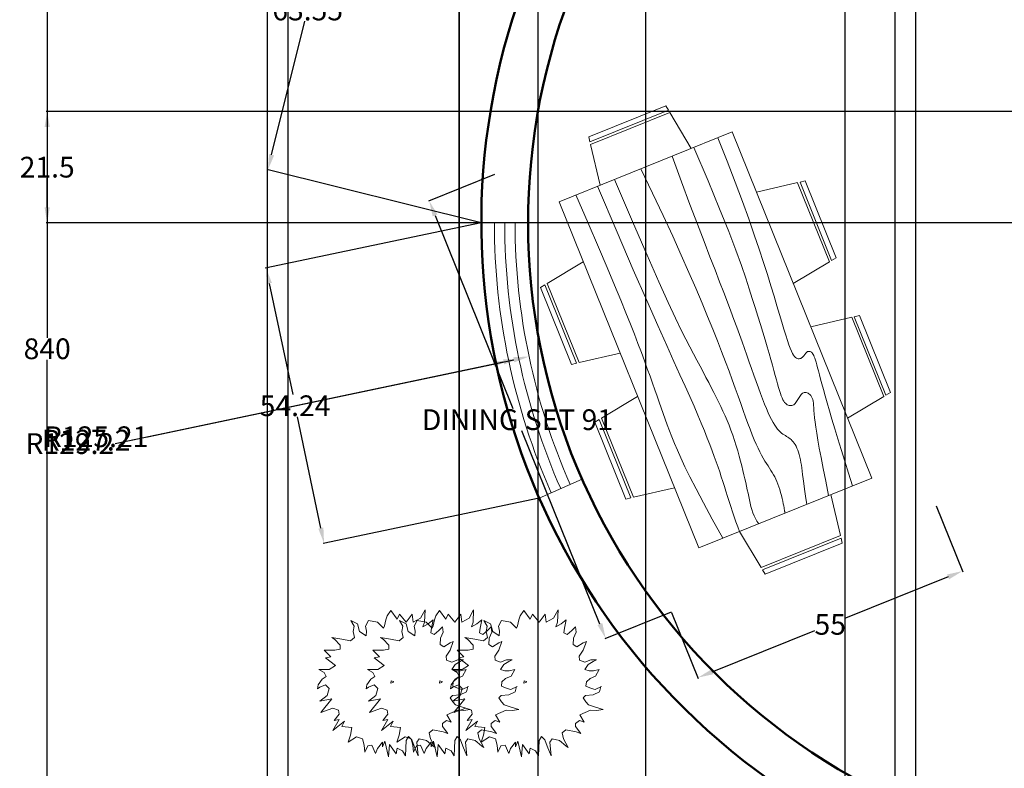
# Model space of a CAD drawing. Units: inches. Extents: x 1331 to 1798, y 701 to 1631.
# Tile 3 of 7: x 1334 to 1524, y 1085 to 1229. Entities that reach past the tile are written whole.
import ezdxf

# ---------------------------------------------------------------- set-up
doc = ezdxf.new("R2010")
doc.units = ezdxf.units.IN
doc.header["$MEASUREMENT"] = 0
for name, color, linetype, lineweight in [('A-ANNO-DIMS', 2, 'Continuous', 18), ('C-PROP', 7, 'Continuous', 25), ('FURNITURE', 18, 'Continuous', 18), ('OUTERWALL', 130, 'Continuous', 50), ('TREES', 102, 'Continuous', 13), ('WINDOWS', 201, 'Continuous', 18)]:
    doc.layers.add(name, color=color, linetype=linetype, lineweight=lineweight)
doc.styles.get("Standard").update_dxf_attribs({"font": 'arial.ttf'})
doc.dimstyles.get("Standard").update_dxf_attribs({"dimtxt": 4, "dimasz": 3, "dimexe": 0.18, "dimexo": 0.0625, "dimgap": 0.09, "dimtad": 0, "dimtih": 1, "dimtoh": 1, "dimdec": 1, "dimzin": 0, "dimdsep": 46, "dimlunit": 3, "dimtxsty": 'Standard', "dimcen": 0.09, "dimadec": 0, "dimazin": 0, "dimtfac": 1, "dimtdec": 1, "dimtofl": 0, "dimtmove": 0, "dimatfit": 3, "dimfxl": 1, "dimtolj": 1, "dimtzin": 0, "dimarcsym": 0})

# ---------------------------------------------------------------- blocks, each defined once
blk = doc.blocks.new('Dining Set - 36 x 72 in.')
for p, q in [((-22, 27.5), (-22.1562, 26.50042)), ((-22, 27.5), (-6, 27.5)), ((-5.8437, 26.49966), (-6, 27.5)), ((6, 27.5), (5.8438, 26.50042)), ((6, 27.5), (22, 27.5)), ((22.1563, 26.49966), (22, 27.5)), ((-22.2343, 26.00059), (-23.4847, 17.99762)), ((-22.2304, 26), (-5.7608, 26)), ((-5.8416, 26.5), (-22.1534, 26.5)), ((-4.5152, 17.99762), (-5.7655, 25.99926)), ((5.7657, 26.00059), (4.5153, 17.99762)), ((5.7696, 26), (22.2392, 26)), ((22.1584, 26.5), (5.8466, 26.5)), ((23.4848, 17.99762), (22.2345, 25.99926)), ((36, 18), (-36, 18)), ((-36, 18), (-36, -18)), ((36, -18), (36, 18)), ((-45.5, 8), (-44.5004, 8.15617)), ((-45.5, 8), (-45.5, -8)), ((-44.5, -8.15843), (-44.5, 8.15338)), ((-44.0006, 8.23428), (-35.9976, 9.48474)), ((-44, 8.23041), (-44, -8.23915)), ((44.0006, 8.23428), (35.9976, 9.48474)), ((44, 8.23041), (44, -8.23915)), ((44.5, -8.15843), (44.5, 8.15338)), ((45.5, 8), (44.5005, 8.15617)), ((45.5, 8), (45.5, -8)), ((-44.4997, -8.15631), (-45.5, -8)), ((-35.9976, -9.48476), (-43.9993, -8.2345)), ((35.9976, -9.48476), (43.9993, -8.2345)), ((44.4997, -8.15631), (45.5, -8)), ((-36, -18), (36, -18)), ((-22.2343, -26.0006), (-23.4847, -17.99762)), ((-4.5152, -17.99762), (-5.7655, -25.99928)), ((5.7657, -26.0006), (4.5153, -17.99762)), ((23.4848, -17.99762), (22.2345, -25.99928)), ((-22.2304, -26), (-5.7608, -26)), ((-22, -27.5), (-22.1562, -26.50044)), ((-5.8416, -26.5), (-22.1534, -26.5)), ((-5.8437, -26.49967), (-6, -27.5)), ((5.7696, -26), (22.2392, -26)), ((6, -27.5), (5.8438, -26.50044)), ((22.1584, -26.5), (5.8466, -26.5)), ((22.1563, -26.49967), (22, -27.5)), ((-22, -27.5), (-6, -27.5)), ((6, -27.5), (22, -27.5))]:
    blk.add_line(p, q)
for points in [[(-36, 15), (-31.1772, 14.97754), (-26.8079, 14.91406), (-22.8538, 14.81543), (-19.276, 14.6875), (-16.0362, 14.53613), (-13.0957, 14.36718), (-10.4159, 14.18652), (-7.9583, 14), (-5.6904, 13.81315), (-3.6035, 13.63021), (-1.6954, 13.45508), (0.0365, 13.29166), (1.5945, 13.14388), (2.9811, 13.01562), (4.1988, 12.9108), (5.25, 12.83333), (6.1393, 12.78613), (6.8802, 12.76823), (7.4883, 12.77767), (7.9792, 12.8125), (8.3685, 12.87077), (8.6719, 12.95052), (8.9049, 13.0498), (9.0833, 13.16666), (9.2205, 13.29899), (9.3216, 13.44401), (9.3895, 13.59879), (9.4271, 13.76041), (9.4373, 13.92594), (9.4232, 14.09245), (9.3875, 14.257), (9.3333, 14.41666), (9.2638, 14.56917), (9.1836, 14.71484), (9.0975, 14.85465), (9.0104, 14.98958), (8.9272, 15.1206), (8.8529, 15.2487), (8.7922, 15.37483), (8.75, 15.5), (8.7305, 15.62467), (8.7344, 15.74739), (8.7617, 15.86621), (8.8125, 15.97916), (8.8867, 16.08431), (8.9844, 16.17968), (9.1055, 16.26334), (9.25, 16.33333), (9.4189, 16.38802), (9.6172, 16.42708), (9.8506, 16.45052), (10.125, 16.45833), (10.4463, 16.45052), (10.8203, 16.42708), (11.2529, 16.38802), (11.75, 16.33333), (12.3184, 16.26318), (12.9694, 16.17838), (13.7151, 16.07991), (14.5677, 15.96875), (15.5395, 15.84586), (16.6426, 15.71224), (17.8893, 15.56884), (19.2917, 15.41666), (20.859, 15.25667), (22.5879, 15.08984), (24.4721, 14.91715), (26.5052, 14.73958), (28.6809, 14.5581), (30.9929, 14.3737), (33.4347, 14.18733), (36, 14)], [(-36, 10), (-28.9766, 10.14274), (-23.1725, 10.20442), (-18.4241, 10.19775), (-14.5677, 10.13541), (-11.4399, 10.03011), (-8.877, 9.89453), (-6.7154, 9.74137), (-4.7917, 9.58333), (-2.9698, 9.43082), (-1.2246, 9.28515), (0.4415, 9.14534), (2.026, 9.01041), (3.5266, 8.87939), (4.9408, 8.7513), (6.266, 8.62516), (7.5, 8.5), (8.6411, 8.37549), (9.6914, 8.2539), (10.6538, 8.13818), (11.5312, 8.03125), (12.3267, 7.93603), (13.043, 7.85547), (13.6831, 7.79248), (14.25, 7.75), (14.7471, 7.7303), (15.1797, 7.73307), (15.5537, 7.75732), (15.875, 7.80208), (16.1494, 7.86637), (16.3828, 7.94922), (16.5811, 8.04964), (16.75, 8.16666), (16.8944, 8.29915), (17.0143, 8.44531), (17.1089, 8.60319), (17.1771, 8.77083), (17.218, 8.94629), (17.2305, 9.1276), (17.2137, 9.31282), (17.1667, 9.5), (17.0895, 9.6875), (16.987, 9.875), (16.8649, 10.0625), (16.7292, 10.25), (16.5856, 10.4375), (16.4401, 10.625), (16.2985, 10.8125), (16.1667, 11), (16.05, 11.18733), (15.9518, 11.3737), (15.8752, 11.5581), (15.8229, 11.73958), (15.798, 11.91715), (15.8034, 12.08984), (15.842, 12.25667), (15.9167, 12.41666), (16.0295, 12.56836), (16.1784, 12.70833), (16.3605, 12.83268), (16.5729, 12.9375), (16.8127, 13.01888), (17.0768, 13.07291), (17.3625, 13.0957), (17.6667, 13.08333), (17.9894, 13.03312), (18.3418, 12.94726), (18.7382, 12.82918), (19.1927, 12.68229), (19.7195, 12.51001), (20.3327, 12.31575), (21.0465, 12.10294), (21.875, 11.875), (22.8357, 11.63354), (23.959, 11.37304), (25.2786, 11.08618), (26.8282, 10.76562), (28.6414, 10.40405), (30.752, 9.99414), (33.1936, 9.52856), (36, 9)], [(-36, 5.5), (-30.7157, 5.3348), (-26.069, 5.20963), (-21.9946, 5.11767), (-18.4271, 5.05208), (-15.3009, 5.00602), (-12.5508, 4.97265), (-10.1112, 4.94515), (-7.9167, 4.91666), (-5.909, 4.88167), (-4.0586, 4.83984), (-2.3429, 4.79215), (-0.7396, 4.73958), (0.7739, 4.6831), (2.22, 4.6237), (3.6213, 4.56233), (5, 4.5), (6.373, 4.43782), (7.7344, 4.3776), (9.0723, 4.32129), (10.375, 4.27083), (11.6309, 4.22819), (12.8281, 4.19531), (13.9551, 4.17415), (15, 4.16666), (15.954, 4.17448), (16.819, 4.19791), (17.6001, 4.23698), (18.3021, 4.29166), (18.9299, 4.36198), (19.4883, 4.44791), (19.9823, 4.54948), (20.4167, 4.66666), (20.7969, 4.79899), (21.1302, 4.94401), (21.4245, 5.09879), (21.6875, 5.26041), (21.9271, 5.42594), (22.1511, 5.59245), (22.3672, 5.757), (22.5834, 5.91666), (22.8065, 6.06868), (23.0404, 6.21093), (23.2879, 6.34147), (23.5521, 6.45833), (23.8358, 6.55957), (24.142, 6.64323), (24.4735, 6.70735), (24.8334, 6.75), (25.2235, 6.76969), (25.642, 6.76692), (26.0858, 6.74267), (26.5521, 6.69791), (27.0379, 6.63362), (27.5404, 6.55078), (28.0565, 6.45036), (28.5834, 6.33333), (29.1242, 6.19987), (29.7071, 6.04687), (30.3661, 5.87044), (31.1354, 5.66666), (32.0493, 5.43164), (33.142, 5.16146), (34.4475, 4.85221), (36, 4.5)], [(-36, -1), (-30.7915, -0.6591), (-26.0195, -0.38216), (-21.6519, -0.16284), (-17.6563, 0.00521), (-14.0005, 0.12833), (-10.6523, 0.21289), (-7.5796, 0.26522), (-4.75, 0.29166), (-2.134, 0.29793), (0.2878, 0.28711), (2.5317, 0.26163), (4.6146, 0.22396), (6.5529, 0.17651), (8.3633, 0.12174), (10.0623, 0.06209), (11.6667, 0), (13.1899, -0.06201), (14.6341, -0.1211), (15.9982, -0.17432), (17.2813, -0.21875), (18.4823, -0.25147), (19.6003, -0.26953), (20.6343, -0.27002), (21.5834, -0.25), (22.4481, -0.20768), (23.2357, -0.14584), (23.9549, -0.06836), (24.6146, 0.02083), (25.2235, 0.11784), (25.7904, 0.21875), (26.3241, 0.31966), (26.8334, 0.41666), (27.3265, 0.50618), (27.8099, 0.58593), (28.2894, 0.65397), (28.7709, 0.70833), (29.2601, 0.74707), (29.763, 0.76823), (30.2855, 0.76985), (30.8334, 0.75), (31.4088, 0.70784), (31.9994, 0.64713), (32.589, 0.57275), (33.1615, 0.48958), (33.7008, 0.4025), (34.1908, 0.3164), (34.6153, 0.23616), (34.9584, 0.16666), (35.2099, 0.11165), (35.3848, 0.07031), (35.504, 0.04069), (35.5886, 0.02083), (35.6594, 0.00879), (35.7377, 0.0026), (35.8442, 0.00032), (36, 0)], [(-36, -6.5), (-27.1843, -6.31267), (-20.084, -6.1263), (-14.469, -5.9419), (-10.1094, -5.76042), (-6.7752, -5.58285), (-4.2363, -5.41016), (-2.2629, -5.24333), (-0.625, -5.08334), (0.8708, -4.93099), (2.2715, -4.78646), (3.5872, -4.64974), (4.8281, -4.52084), (6.0046, -4.39974), (7.127, -4.28646), (8.2053, -4.18099), (9.25, -4.08334), (10.2705, -3.99382), (11.2734, -3.91407), (12.2647, -3.84603), (13.25, -3.79167), (14.2354, -3.75293), (15.2266, -3.73177), (16.2295, -3.73015), (17.25, -3.75), (18.2912, -3.79248), (19.3451, -3.85547), (20.4009, -3.93604), (21.4479, -4.03125), (22.4754, -4.13819), (23.4727, -4.25391), (24.4289, -4.37549), (25.3334, -4.5), (26.1785, -4.62492), (26.9694, -4.74935), (27.7145, -4.87281), (28.4219, -4.99479), (29.1, -5.11483), (29.7572, -5.23242), (30.4016, -5.34709), (31.0417, -5.45834), (31.6837, -5.56437), (32.3262, -5.65821), (32.9658, -5.73153), (33.599, -5.77604), (34.2224, -5.78345), (34.8327, -5.74545), (35.4264, -5.65373), (36, -5.5)], [(-36, -10), (-26.4022, -9.81299), (-18.4675, -9.62891), (-11.9839, -9.45069), (-6.7396, -9.28125), (-2.5226, -9.12354), (0.8789, -8.98047), (3.6769, -8.85498), (6.0833, -8.75), (8.2767, -8.66765), (10.3021, -8.60677), (12.1712, -8.56543), (13.8958, -8.54167), (15.4876, -8.53353), (16.9583, -8.53907), (18.3197, -8.55632), (19.5834, -8.58334), (20.7616, -8.61841), (21.8685, -8.66081), (22.9188, -8.71004), (23.9271, -8.76563), (24.9081, -8.82707), (25.8763, -8.89388), (26.8465, -8.96558), (27.8334, -9.04167), (28.8474, -9.12118), (29.8828, -9.20117), (30.93, -9.27824), (31.9792, -9.34896), (33.0205, -9.40991), (34.0443, -9.45768), (35.0407, -9.48885), (36, -9.5)], [(-36, -14.5), (-30.0881, -14.33513), (-25.0332, -14.21224), (-20.7312, -14.12647), (-17.0781, -14.07292), (-13.97, -14.04671), (-11.3027, -14.04297), (-8.9724, -14.05681), (-6.875, -14.08334), (-4.9224, -14.11833), (-3.0905, -14.16016), (-1.3709, -14.20785), (0.2448, -14.26042), (1.7647, -14.3169), (3.1973, -14.3763), (4.5507, -14.43767), (5.8333, -14.5), (7.0554, -14.5621), (8.235, -14.62175), (9.3922, -14.67652), (10.5469, -14.72396), (11.7192, -14.76164), (12.929, -14.78711), (14.1965, -14.79794), (15.5417, -14.79167), (16.9933, -14.76424), (18.6152, -14.70508), (20.4804, -14.60197), (22.6615, -14.44271), (25.2312, -14.21509), (28.2624, -13.9069), (31.8277, -13.50594), (36, -13)]]:
    blk.add_lwpolyline(points)
blk = doc.blocks.new('*U9')
for points in [[(0, 1540.256), (-77.4954, 1428.4452), (-106.5784, 1341.501), (-135.636, 1217.295), (-155.0162, 1167.6126), (-280.9748, 1291.8186), (-474.7514, 1329.0804), (-532.892, 1204.8744), (-513.5118, 1105.5096), (-523.1892, 1006.1194), (-658.8506, 1093.089), (-707.2884, 1254.5568), (-842.9244, 1329.0804), (-775.1064, 1204.8744), (-794.4866, 1093.089), (-765.429, 968.8576), (-852.6272, 894.334), (-1036.701, 931.5958), (-1249.8832, 968.8576), (-1191.7426, 931.5958), (-1075.4614, 807.3898), (-1075.4614, 720.4456), (-1182.0398, 695.6044), (-1414.5768, 695.6044), (-1269.238, 558.9524), (-1385.5192, 534.1112), (-1172.3624, 372.6434), (-1307.9984, 285.6992), (-1521.1552, 285.6992), (-1414.5768, 223.5962), (-1366.139, 136.652), (-1453.3372, 86.9442), (-1540.5354, -37.2618), (-1550.2382, -124.206), (-1501.775, -86.9442), (-1385.5192, -37.2618), (-1307.9984, -111.7854), (-1346.7588, -260.8326), (-1501.775, -385.064), (-1249.8832, -335.3816), (-1482.3948, -621.0554), (-1230.503, -534.1112), (-1104.5444, -571.373), (-1094.8416, -658.3172), (-1201.42, -794.9692), (-1094.8416, -770.128), (-1230.503, -1006.1194), (-978.5858, -807.3898), (-1036.701, -919.1752), (-823.5442, -944.0164), (-852.6272, -1105.4842), (-901.065, -1254.5568), (-726.6686, -1142.746), (-600.71, -1180.0078), (-561.9496, -1316.6598), (-552.2722, -1465.707), (-484.4542, -1329.0804), (-397.2306, -1316.6598), (-319.7352, -1490.5482), (-280.9748, -1391.1834), (-174.3964, -1254.5568), (-174.3964, -1353.9216), (-125.9586, -1229.7156), (-48.4378, -1565.0718), (-29.0576, -1304.2392), (116.2812, -1502.9688), (135.6614, -1378.7628), (251.9172, -1440.8658), (310.0578, -1540.2306), (329.438, -1217.295), (377.8758, -1130.3254), (445.6938, -1204.8744), (494.157, -1341.501), (581.3552, -1540.2306), (552.2722, -1254.5568), (600.71, -1180.0078), (755.7516, -1217.295), (891.3876, -1329.0804), (939.8254, -1366.3422), (842.9498, -1180.0078), (813.8668, -1055.8018), (891.3876, -993.6988), (1114.2472, -1030.9606), (1211.1228, -1068.2224), (1094.867, -919.1752), (1094.867, -857.0722), (1182.0652, -794.9692), (1278.9408, -832.231), (1191.7426, -670.7378), (1414.6022, -571.373), (1540.5608, -583.7936), (1685.8996, -558.9524), (1521.1806, -509.27), (1375.8418, -459.5876), (1317.7012, -397.4846), (1259.5606, -310.515), (1308.0238, -260.8326), (1472.7174, -248.412), (1608.3788, -186.309), (1637.4364, -74.5236)], [(1647.1392, -74.5236), (1511.4778, -136.6266), (1433.9824, -111.7854), (1317.7012, -62.103), (1327.404, 24.8412), (1404.8994, 99.3648), (1521.1806, 149.0726), (1598.676, 285.6992), (1482.4202, 260.858), (1385.5192, 260.858), (1298.321, 285.6992), (1366.139, 397.4846), (1472.7174, 459.5876), (1540.5608, 496.8494), (1424.2796, 496.8494), (1298.321, 447.167), (1182.0652, 484.4288), (1172.3624, 571.3984), (1259.5606, 695.6044), (1327.404, 881.9134), (1259.5606, 857.0722), (1123.9246, 770.128), (1046.4038, 819.8104), (1056.1066, 956.437), (1114.2472, 1080.6684), (1094.867, 1192.4538), (1017.3462, 1117.9302), (920.4452, 1030.9606), (852.6272, 1068.2478), (862.33, 1167.6126), (901.0904, 1341.501), (794.512, 1254.5568), (678.2308, 1192.4538), (716.9912, 1291.8186), (726.6686, 1552.6766), (629.793, 1378.7628), (474.7768, 1291.8186), (455.3966, 1465.7324), (329.438, 1291.8186), (184.0992, 1465.7324), (135.6614, 1353.9216), (0, 1540.256)]]:
    blk.add_lwpolyline(points)
blk.add_lwpolyline([(9.7028, 49.6824), (0, 0), (48.4378, 12.4206), (58.1406, 37.2618)], close=True)
blk = doc.blocks.new('*D42')
at = {"layer": 'A-ANNO-DIMS', "color": 0, "lineweight": -2, "transparency": 16777216}
for p, q in [((1425.5, 1199.53), (1412.73, 1194.38)), ((1414.02, 1191.67), (1429.04, 1154.41)), ((1445.79, 1112.83), (1430.78, 1150.09)), ((1459.52, 1115.13), (1446.75, 1109.98))]:
    blk.add_line(p, q, dxfattribs=at)
at = {"layer": 'A-ANNO-DIMS', "color": 0, "transparency": 16777216}
for points in [[(1414.48, 1191.85), (1413.56, 1191.48), (1412.9, 1194.45)], [(1446.26, 1113.02), (1445.33, 1112.64), (1446.92, 1110.05)]]:
    blk.add_solid(points, dxfattribs=at)
at = {"layer": 'Defpoints', "color": 0, "transparency": 16777216}
for p in [(1425.56, 1199.55), (1459.58, 1115.15), (1446.92, 1110.05)]:
    blk.add_point(p, dxfattribs=at)
at = {"layer": 'A-ANNO-DIMS', "color": 0, "transparency": 16777216, "insert": (1429.91, 1152.25), "char_height": 4, "attachment_point": 5}
blk.add_mtext('\\A1;DINING SET 91', dxfattribs=at)
blk = doc.blocks.new('*D43')
at = {"layer": 'A-ANNO-DIMS', "color": 0, "lineweight": -2, "transparency": 16777216}
for p, q in [((1510.61, 1135.65), (1515.76, 1122.88)), ((1512.91, 1121.93), (1493.16, 1113.97)), ((1459.6, 1115.09), (1464.75, 1102.32)), ((1467.46, 1103.61), (1487.22, 1111.57))]:
    blk.add_line(p, q, dxfattribs=at)
at = {"layer": 'A-ANNO-DIMS', "color": 0, "transparency": 16777216}
for points in [[(1512.72, 1122.39), (1513.1, 1121.46), (1515.69, 1123.05)], [(1467.27, 1104.07), (1467.65, 1103.15), (1464.68, 1102.49)]]:
    blk.add_solid(points, dxfattribs=at)
at = {"layer": 'Defpoints', "color": 0, "transparency": 16777216}
for p in [(1510.59, 1135.71), (1515.69, 1123.05), (1459.58, 1115.15)]:
    blk.add_point(p, dxfattribs=at)
at = {"layer": 'A-ANNO-DIMS', "color": 0, "transparency": 16777216, "insert": (1490.19, 1112.77), "char_height": 4, "attachment_point": 5}
blk.add_mtext('\\A1;55', dxfattribs=at)
blk = doc.blocks.new('*D51')
at = {"layer": 'A-ANNO-DIMS', "color": 0, "lineweight": -2, "transparency": 16777216}
for p, q in [((1381.6, 1585.93), (1339.08, 1585.93)), ((1339.26, 1582.93), (1339.26, 1168.06)), ((1339.26, 748.93), (1339.26, 1163.79)), ((1381.6, 745.93), (1339.08, 745.93))]:
    blk.add_line(p, q, dxfattribs=at)
at = {"layer": 'A-ANNO-DIMS', "color": 0, "transparency": 16777216}
for points in [[(1338.76, 1582.93), (1339.76, 1582.93), (1339.26, 1585.93)], [(1338.76, 748.93), (1339.76, 748.93), (1339.26, 745.93)]]:
    blk.add_solid(points, dxfattribs=at)
at = {"layer": 'Defpoints', "color": 0, "transparency": 16777216}
for p in [(1339.26, 1585.93), (1381.66, 1585.93), (1381.66, 745.93)]:
    blk.add_point(p, dxfattribs=at)
at = {"layer": 'A-ANNO-DIMS', "color": 0, "transparency": 16777216, "insert": (1339.26, 1165.93), "char_height": 4, "attachment_point": 5}
blk.add_mtext('\\A1;840', dxfattribs=at)
blk = doc.blocks.new('*D60')
at = {"layer": 'A-ANNO-DIMS', "color": 0, "lineweight": -2, "transparency": 16777216}
for p, q in [((1418.66, 1524.86), (1418.66, 703.35)), ((1433.85, 1524.86), (1433.85, 703.35)), ((1421.66, 703.53), (1430.85, 703.53)), ((1433.85, 703.53), (1436.85, 703.53))]:
    blk.add_line(p, q, dxfattribs=at)
at = {"layer": 'A-ANNO-DIMS', "color": 0, "transparency": 16777216}
for points in [[(1421.66, 704.03), (1421.66, 703.03), (1418.66, 703.53)], [(1430.85, 704.03), (1430.85, 703.03), (1433.85, 703.53)]]:
    blk.add_solid(points, dxfattribs=at)
at = {"layer": 'Defpoints', "color": 0, "transparency": 16777216}
for p in [(1418.66, 1524.93), (1433.85, 1524.93), (1433.85, 703.53)]:
    blk.add_point(p, dxfattribs=at)
at = {"layer": 'A-ANNO-DIMS', "color": 0, "transparency": 16777216, "insert": (1445.06, 703.53), "char_height": 4, "attachment_point": 5}
blk.add_mtext('\\A1;15.188', dxfattribs=at)
blk = doc.blocks.new('*D67')
at = {"layer": 'A-ANNO-DIMS', "color": 0, "lineweight": -2, "transparency": 16777216}
for p, q in [((1418.66, 1316.86), (1418.66, 703.35)), ((1502.66, 1316.86), (1502.66, 703.35)), ((1421.66, 703.53), (1457.71, 703.53)), ((1499.66, 703.53), (1463.61, 703.53))]:
    blk.add_line(p, q, dxfattribs=at)
at = {"layer": 'A-ANNO-DIMS', "color": 0, "transparency": 16777216}
for points in [[(1421.66, 704.03), (1421.66, 703.03), (1418.66, 703.53)], [(1499.66, 704.03), (1499.66, 703.03), (1502.66, 703.53)]]:
    blk.add_solid(points, dxfattribs=at)
at = {"layer": 'Defpoints', "color": 0, "transparency": 16777216}
for p in [(1418.66, 1316.93), (1502.66, 1316.93), (1502.66, 703.53)]:
    blk.add_point(p, dxfattribs=at)
at = {"layer": 'A-ANNO-DIMS', "color": 0, "transparency": 16777216, "insert": (1460.66, 703.53), "char_height": 4, "attachment_point": 5}
blk.add_mtext('\\A1;84', dxfattribs=at)
blk = doc.blocks.new('*D71')
at = {"layer": 'A-ANNO-DIMS', "color": 0, "lineweight": -2, "transparency": 16777216}
for p, q in [((1506.66, 1376.86), (1506.66, 703.35)), ((1610.66, 1376.86), (1610.66, 703.35)), ((1509.66, 703.53), (1554.35, 703.53)), ((1607.66, 703.53), (1562.98, 703.53))]:
    blk.add_line(p, q, dxfattribs=at)
at = {"layer": 'A-ANNO-DIMS', "color": 0, "transparency": 16777216}
for points in [[(1509.66, 704.03), (1509.66, 703.03), (1506.66, 703.53)], [(1607.66, 704.03), (1607.66, 703.03), (1610.66, 703.53)]]:
    blk.add_solid(points, dxfattribs=at)
at = {"layer": 'Defpoints', "color": 0, "transparency": 16777216}
for p in [(1506.66, 1376.93), (1610.66, 1376.93), (1610.66, 703.53)]:
    blk.add_point(p, dxfattribs=at)
at = {"layer": 'A-ANNO-DIMS', "color": 0, "transparency": 16777216, "insert": (1558.66, 703.53), "char_height": 4, "attachment_point": 5}
blk.add_mtext('\\A1;104', dxfattribs=at)
blk = doc.blocks.new('*D81')
at = {"layer": 'A-ANNO-DIMS', "color": 0, "lineweight": -2, "transparency": 16777216}
for p, q in [((1418.66, 941.85), (1418.66, 1628.51)), ((1493.07, 941.85), (1493.07, 1628.51)), ((1421.66, 1628.33), (1449.43, 1628.33)), ((1490.07, 1628.33), (1462.3, 1628.33))]:
    blk.add_line(p, q, dxfattribs=at)
at = {"layer": 'A-ANNO-DIMS', "color": 0, "transparency": 16777216}
for points in [[(1421.66, 1628.83), (1421.66, 1627.83), (1418.66, 1628.33)], [(1490.07, 1628.83), (1490.07, 1627.83), (1493.07, 1628.33)]]:
    blk.add_solid(points, dxfattribs=at)
at = {"layer": 'Defpoints', "color": 0, "transparency": 16777216}
for p in [(1493.07, 1628.33), (1418.66, 941.79), (1493.07, 941.79)]:
    blk.add_point(p, dxfattribs=at)
at = {"layer": 'A-ANNO-DIMS', "color": 0, "transparency": 16777216, "insert": (1455.87, 1628.33), "char_height": 4, "attachment_point": 5}
blk.add_mtext('\\A1;74.41', dxfattribs=at)
blk = doc.blocks.new('*D83')
at = {"layer": 'A-ANNO-DIMS', "color": 0, "lineweight": -2, "transparency": 16777216}
for p, q in [((1418.66, 1022.23), (1418.66, 1628.51)), ((1454.66, 1022.23), (1454.66, 1628.51)), ((1421.66, 1628.33), (1433.71, 1628.33)), ((1451.66, 1628.33), (1439.62, 1628.33))]:
    blk.add_line(p, q, dxfattribs=at)
at = {"layer": 'A-ANNO-DIMS', "color": 0, "transparency": 16777216}
for points in [[(1421.66, 1628.83), (1421.66, 1627.83), (1418.66, 1628.33)], [(1451.66, 1628.83), (1451.66, 1627.83), (1454.66, 1628.33)]]:
    blk.add_solid(points, dxfattribs=at)
at = {"layer": 'Defpoints', "color": 0, "transparency": 16777216}
for p in [(1454.66, 1628.33), (1418.66, 1022.17), (1454.66, 1022.17)]:
    blk.add_point(p, dxfattribs=at)
at = {"layer": 'A-ANNO-DIMS', "color": 0, "transparency": 16777216, "insert": (1436.66, 1628.33), "char_height": 4, "attachment_point": 5}
blk.add_mtext('\\A1;36', dxfattribs=at)
blk = doc.blocks.new('*D90')
at = {"layer": 'A-ANNO-DIMS', "color": 0, "lineweight": -2, "transparency": 16777216}
for p, q in [((1554.66, 1190.15), (1554.66, 703.35)), ((1409.66, 805.73), (1409.66, 703.35)), ((1412.66, 703.53), (1477.83, 703.53)), ((1551.66, 703.53), (1486.5, 703.53))]:
    blk.add_line(p, q, dxfattribs=at)
at = {"layer": 'A-ANNO-DIMS', "color": 0, "transparency": 16777216}
for points in [[(1412.66, 704.03), (1412.66, 703.03), (1409.66, 703.53)], [(1551.66, 704.03), (1551.66, 703.03), (1554.66, 703.53)]]:
    blk.add_solid(points, dxfattribs=at)
at = {"layer": 'Defpoints', "color": 0, "transparency": 16777216}
for p in [(1554.66, 1190.21), (1409.66, 805.79), (1554.66, 703.53)]:
    blk.add_point(p, dxfattribs=at)
at = {"layer": 'A-ANNO-DIMS', "color": 0, "transparency": 16777216, "insert": (1482.16, 703.53), "char_height": 4, "attachment_point": 5}
blk.add_mtext('\\A1;145', dxfattribs=at)
blk = doc.blocks.new('*D93')
at = {"layer": 'A-ANNO-DIMS', "color": 0, "lineweight": -2, "transparency": 16777216}
for p, q in [((1422.89, 1190.2), (1381.28, 1181.45)), ((1382.08, 1178.55), (1386.59, 1157.08)), ((1392.01, 1131.34), (1387.49, 1152.81)), ((1434.06, 1137.12), (1392.45, 1128.37))]:
    blk.add_line(p, q, dxfattribs=at)
at = {"layer": 'A-ANNO-DIMS', "color": 0, "transparency": 16777216}
for points in [[(1382.57, 1178.65), (1381.59, 1178.44), (1381.46, 1181.48)], [(1392.5, 1131.44), (1391.52, 1131.24), (1392.63, 1128.4)]]:
    blk.add_solid(points, dxfattribs=at)
at = {"layer": 'Defpoints', "color": 0, "transparency": 16777216}
for p in [(1422.95, 1190.21), (1381.46, 1181.48), (1434.12, 1137.14)]:
    blk.add_point(p, dxfattribs=at)
at = {"layer": 'A-ANNO-DIMS', "color": 0, "transparency": 16777216, "insert": (1387.04, 1154.94), "char_height": 4, "attachment_point": 5}
blk.add_mtext('\\A1;54.24', dxfattribs=at)
blk = doc.blocks.new('*D94')
at = {"layer": 'A-ANNO-DIMS', "color": 0, "lineweight": -2, "transparency": 16777216}
for p, q in [((1438.22, 1251.9), (1396.96, 1262.16)), ((1396.41, 1259.2), (1390, 1233.41)), ((1382.53, 1203.35), (1388.94, 1229.15)), ((1422.89, 1190.23), (1381.63, 1200.49))]:
    blk.add_line(p, q, dxfattribs=at)
at = {"layer": 'A-ANNO-DIMS', "color": 0, "transparency": 16777216}
for points in [[(1395.93, 1259.32), (1396.9, 1259.08), (1397.13, 1262.12)], [(1382.04, 1203.47), (1383.01, 1203.23), (1381.8, 1200.44)]]:
    blk.add_solid(points, dxfattribs=at)
at = {"layer": 'Defpoints', "color": 0, "transparency": 16777216}
for p in [(1397.13, 1262.12), (1438.28, 1251.89), (1422.95, 1190.21)]:
    blk.add_point(p, dxfattribs=at)
at = {"layer": 'A-ANNO-DIMS', "color": 0, "transparency": 16777216, "insert": (1389.47, 1231.28), "char_height": 4, "attachment_point": 5}
blk.add_mtext('\\A1;63.55', dxfattribs=at)
blk = doc.blocks.new('*D97')
at = {"layer": 'A-ANNO-DIMS', "color": 0, "lineweight": -2, "transparency": 16777216}
for p, q in [((1684.55, 1211.71), (1339.08, 1211.71)), ((1339.26, 1208.71), (1339.26, 1203.1)), ((1339.26, 1193.21), (1339.26, 1198.83)), ((1554.6, 1190.21), (1339.08, 1190.21))]:
    blk.add_line(p, q, dxfattribs=at)
at = {"layer": 'A-ANNO-DIMS', "color": 0, "transparency": 16777216}
for points in [[(1338.76, 1208.71), (1339.76, 1208.71), (1339.26, 1211.71)], [(1338.76, 1193.21), (1339.76, 1193.21), (1339.26, 1190.21)]]:
    blk.add_solid(points, dxfattribs=at)
at = {"layer": 'Defpoints', "color": 0, "transparency": 16777216}
for p in [(1684.61, 1211.71), (1339.26, 1190.21), (1554.66, 1190.21)]:
    blk.add_point(p, dxfattribs=at)
at = {"layer": 'A-ANNO-DIMS', "color": 0, "transparency": 16777216, "insert": (1339.26, 1200.96), "char_height": 4, "attachment_point": 5}
blk.add_mtext('\\A1;21.5', dxfattribs=at)
blk = doc.blocks.new('*D100')
at = {"layer": 'A-ANNO-DIMS', "color": 0, "lineweight": -2, "transparency": 16777216}
for p, q in [((1395.06, 1326.62), (1398.06, 1326.62)), ((1398.06, 1326.62), (1454.52, 1277.44)), ((1554.57, 1190.21), (1554.75, 1190.21)), ((1554.66, 1190.12), (1554.66, 1190.3))]:
    blk.add_line(p, q, dxfattribs=at)
at = {"layer": 'A-ANNO-DIMS', "color": 0, "transparency": 16777216}
blk.add_solid([(1454.85, 1277.81), (1454.19, 1277.06), (1456.78, 1275.47)], dxfattribs=at)
at = {"layer": 'Defpoints', "color": 0, "transparency": 16777216}
for p in [(1456.78, 1275.47), (1554.66, 1190.21)]:
    blk.add_point(p, dxfattribs=at)
at = {"layer": 'A-ANNO-DIMS', "color": 0, "transparency": 16777216, "insert": (1386.3, 1326.62), "char_height": 4, "attachment_point": 5}
blk.add_mtext('\\A1;R129.8', dxfattribs=at)
blk = doc.blocks.new('*D101')
at = {"layer": 'A-ANNO-DIMS', "color": 0, "lineweight": -2, "transparency": 16777216}
for p, q in [((1554.57, 1190.21), (1554.75, 1190.21)), ((1554.66, 1190.12), (1554.66, 1190.3)), ((1352.35, 1147.64), (1425.28, 1162.99))]:
    blk.add_line(p, q, dxfattribs=at)
at = {"layer": 'A-ANNO-DIMS', "color": 0, "transparency": 16777216}
blk.add_solid([(1425.18, 1163.48), (1425.39, 1162.5), (1428.22, 1163.61)], dxfattribs=at)
at = {"layer": 'Defpoints', "color": 0, "transparency": 16777216}
for p in [(1554.66, 1190.21), (1428.22, 1163.61)]:
    blk.add_point(p, dxfattribs=at)
at = {"layer": 'A-ANNO-DIMS', "color": 0, "transparency": 16777216, "insert": (1343.62, 1147.64), "char_height": 4, "attachment_point": 5}
blk.add_mtext('\\A1;R129.2', dxfattribs=at)
blk = doc.blocks.new('*D103')
at = {"layer": 'A-ANNO-DIMS', "color": 0, "lineweight": -2, "transparency": 16777216}
for p, q in [((1554.57, 1190.21), (1554.75, 1190.21)), ((1554.66, 1190.12), (1554.66, 1190.3)), ((1355.48, 1148.3), (1427.24, 1163.4))]:
    blk.add_line(p, q, dxfattribs=at)
at = {"layer": 'A-ANNO-DIMS', "color": 0, "transparency": 16777216}
blk.add_solid([(1427.14, 1163.89), (1427.34, 1162.91), (1430.18, 1164.02)], dxfattribs=at)
at = {"layer": 'Defpoints', "color": 0, "transparency": 16777216}
for p in [(1554.66, 1190.21), (1430.18, 1164.02)]:
    blk.add_point(p, dxfattribs=at)
at = {"layer": 'A-ANNO-DIMS', "color": 0, "transparency": 16777216, "insert": (1346.75, 1148.3), "char_height": 4, "attachment_point": 5}
blk.add_mtext('\\A1;R127.2', dxfattribs=at)
blk = doc.blocks.new('*D105')
at = {"layer": 'A-ANNO-DIMS', "color": 0, "lineweight": -2, "transparency": 16777216}
for p, q in [((1554.57, 1190.21), (1554.75, 1190.21)), ((1554.66, 1190.12), (1554.66, 1190.3)), ((1358.62, 1148.96), (1429.2, 1163.81))]:
    blk.add_line(p, q, dxfattribs=at)
at = {"layer": 'A-ANNO-DIMS', "color": 0, "transparency": 16777216}
blk.add_solid([(1429.1, 1164.3), (1429.3, 1163.32), (1432.13, 1164.43)], dxfattribs=at)
at = {"layer": 'Defpoints', "color": 0, "transparency": 16777216}
for p in [(1554.66, 1190.21), (1432.13, 1164.43)]:
    blk.add_point(p, dxfattribs=at)
at = {"layer": 'A-ANNO-DIMS', "color": 0, "transparency": 16777216, "insert": (1348.7, 1148.96), "char_height": 4, "attachment_point": 5}
blk.add_mtext('\\A1;R125.21', dxfattribs=at)
blk = doc.blocks.new('*D107')
at = {"layer": 'A-ANNO-DIMS', "color": 0, "lineweight": -2, "transparency": 16777216}
for p, q in [((1400.92, 1320.71), (1403.92, 1320.71)), ((1403.92, 1320.71), (1458.18, 1273.74)), ((1554.57, 1190.21), (1554.75, 1190.21)), ((1554.66, 1190.12), (1554.66, 1190.3))]:
    blk.add_line(p, q, dxfattribs=at)
at = {"layer": 'A-ANNO-DIMS', "color": 0, "transparency": 16777216}
blk.add_solid([(1458.51, 1274.11), (1457.85, 1273.36), (1460.45, 1271.77)], dxfattribs=at)
at = {"layer": 'Defpoints', "color": 0, "transparency": 16777216}
for p in [(1460.45, 1271.77), (1554.66, 1190.21)]:
    blk.add_point(p, dxfattribs=at)
at = {"layer": 'A-ANNO-DIMS', "color": 0, "transparency": 16777216, "insert": (1392.17, 1320.71), "char_height": 4, "attachment_point": 5}
blk.add_mtext('\\A1;R124.6', dxfattribs=at)

msp = doc.modelspace()

# ---------------------------------------------------------------- linework, layer by layer
at = {"layer": 'C-PROP'}
msp.add_line((1385.6637, 1581.9256), (1385.6637, 749.9256), dxfattribs=at)
msp.add_lwpolyline([(1737.6637, 745.9256), (1741.6637, 745.9256), (1741.6637, 1585.9256), (1381.6637, 1585.9256), (1381.6637, 745.9256), (1559.6637, 745.9256)], dxfattribs=at)
msp.add_lwpolyline([(1737.6637, 745.9256), (1741.6637, 745.9256), (1741.6637, 1585.9256), (1381.6637, 1585.9256), (1381.6637, 745.9256), (1559.6637, 745.9256)], dxfattribs=at)
at = {"layer": 'OUTERWALL'}
for radius, start, end in [(131.7127, 152.079594, 234.646719), (122.7127, 153.37533, 243.419216)]:
    msp.add_arc((1554.6637, 1190.2129), radius, start, end, dxfattribs=at)
at = {"layer": 'WINDOWS'}
for p, q in [((1422.951, 1190.2129), (1431.951, 1190.2129)), ((1434.1192, 1137.1351), (1442.3561, 1140.7619))]:
    msp.add_line(p, q, dxfattribs=at)
for radius in [129.2127, 127.2127, 125.2127]:
    msp.add_arc((1554.6637, 1190.2129), radius, 180, 203.764719, dxfattribs=at)

# ---------------------------------------------------------------- block references
at = {"layer": 'FURNITURE', "rotation": 291.9512548559181}
msp.add_blockref('Dining Set - 36 x 72 in.', (1468.0739, 1167.6308), dxfattribs=at)
at = {"layer": 'TREES', "xscale": 0.0090900995059179, "yscale": 0.0090900995059179, "zscale": 0.0090900995059179}
for p in [(1405.4799, 1101.4406), (1414.86, 1101.4406), (1431.1188, 1101.4406)]:
    msp.add_blockref('*U9', p, dxfattribs=at)

# ---------------------------------------------------------------- dimensions: what is measured, and where the dimension line sits
at = {"layer": 'A-ANNO-DIMS'}
for base, p1, p2, override, picture, middle in [((1493.0724, 1628.3256), (1418.6637, 941.7881), (1493.0724, 941.7881), {"dimdec": 2, "dimlfac": 1, "dimrnd": 0, "dimzin": 0, "dimdsep": 46, "dimlunit": 2}, '*D81', (1455.8681, 1628.3256)), ((1454.6637, 1628.3256), (1418.6637, 1022.1692), (1454.6637, 1022.1692), {"dimdec": 0, "dimlfac": 1, "dimrnd": 0, "dimzin": 0, "dimdsep": 46, "dimlunit": 2}, '*D83', (1436.6637, 1628.3256)), ((1433.8519, 703.5256), (1418.6637, 1524.9256), (1433.8519, 1524.9256), {"dimdec": 3, "dimlfac": 1, "dimrnd": 0, "dimzin": 0, "dimdsep": 46, "dimlunit": 2}, '*D60', (1445.0606, 703.5256)), ((1610.6637, 703.5256), (1506.6637, 1376.9256), (1610.6637, 1376.9256), {"dimdec": 0, "dimlfac": 1, "dimrnd": 0, "dimzin": 0, "dimdsep": 46, "dimlunit": 2}, '*D71', (1558.6637, 703.5256)), ((1502.6637, 703.5256), (1418.6637, 1316.9256), (1502.6637, 1316.9256), {"dimdec": 0, "dimlfac": 1, "dimrnd": 0, "dimzin": 0, "dimdsep": 46, "dimlunit": 2}, '*D67', (1460.6637, 703.5256)), ((1554.6637, 703.5256), (1409.6637, 805.7881), (1554.6637, 1190.2129), {"dimdec": 0, "dimlfac": 1, "dimrnd": 0, "dimzin": 0, "dimdsep": 46, "dimlunit": 2}, '*D90', (1482.1637, 703.5256))]:
    dim = msp.add_linear_dim(base=base, p1=p1, p2=p2, dimstyle='Standard', override=override, dxfattribs=at)
    dim.commit()
    dim.dimension.update_dxf_attribs({"geometry": picture, "text_midpoint": middle})
for base, p1, p2, angle, override, picture, middle in [((1339.2637, 1585.9256), (1381.6637, 745.9256), (1381.6637, 1585.9256), 90, {"dimdec": 0, "dimlfac": 1, "dimrnd": 0, "dimzin": 0, "dimdsep": 46, "dimlunit": 2}, '*D51', (1339.2637, 1165.9256)), ((1397.1349, 1262.1156), (1422.951, 1190.2129), (1438.2825, 1251.8867), 76.039797, {"dimdec": 2, "dimlfac": 1, "dimrnd": 0, "dimzin": 0, "dimdsep": 46, "dimlunit": 2}, '*D94', (1389.4691, 1231.2787)), ((1339.2637, 1190.2129), (1684.6094, 1211.7148), (1554.6637, 1190.2129), 90, {"dimdec": 1, "dimlfac": 1, "dimrnd": 0, "dimzin": 0, "dimdsep": 46, "dimlunit": 2}, '*D97', (1339.2637, 1200.9639)), ((1381.4596, 1181.4826), (1434.1192, 1137.1351), (1422.951, 1190.2129), 101.882359, {"dimdec": 2, "dimlfac": 1, "dimrnd": 0, "dimzin": 0, "dimdsep": 46, "dimlunit": 2}, '*D93', (1387.0436, 1154.9437)), ((1515.6916, 1123.049), (1459.5763, 1115.1495), (1510.589, 1135.7094), 21.951255, {"dimdec": 0, "dimlfac": 1, "dimrnd": 0, "dimzin": 0, "dimdsep": 46, "dimlunit": 2}, '*D43', (1490.1853, 1112.769))]:
    dim = msp.add_linear_dim(base=base, p1=p1, p2=p2, angle=angle, dimstyle='Standard', override=override, dxfattribs=at)
    dim.commit()
    dim.dimension.update_dxf_attribs({"geometry": picture, "text_midpoint": middle})
for mpoint, override, picture, middle in [((1456.7847, 1275.4673), {"dimdec": 1, "dimlfac": 1, "dimrnd": 0, "dimzin": 0, "dimdsep": 46, "dimlunit": 2}, '*D100', (1386.3001, 1326.6199)), ((1460.4492, 1271.7718), {"dimdec": 1, "dimlfac": 1, "dimrnd": 0, "dimzin": 0, "dimdsep": 46, "dimlunit": 2}, '*D107', (1392.1689, 1320.7071)), ((1428.2197, 1163.6079), {"dimdec": 1, "dimlfac": 1, "dimrnd": 0, "dimzin": 0, "dimdsep": 46, "dimlunit": 2}, '*D101', (1352.3533, 1147.6449)), ((1430.177, 1164.019), {"dimdec": 1, "dimlfac": 1, "dimrnd": 0, "dimzin": 0, "dimdsep": 46, "dimlunit": 2}, '*D103', (1355.485, 1148.3026)), ((1432.1341, 1164.431), {"dimdec": 2, "dimlfac": 1, "dimrnd": 0, "dimzin": 0, "dimdsep": 46, "dimlunit": 2}, '*D105', (1358.6163, 1148.9619))]:
    dim = msp.add_radius_dim(center=(1554.6637, 1190.2129), mpoint=mpoint, dimstyle='Standard', override=override, dxfattribs=at)
    dim.commit()
    dim.dimension.update_dxf_attribs({"geometry": picture, "text_midpoint": middle, "dimtype": 164})
dim = msp.add_linear_dim(base=(1446.9159, 1110.0469), p1=(1425.5589, 1199.5522), p2=(1459.5763, 1115.1495), angle=291.951255, text='DINING SET <>', dimstyle='Standard', override={"dimdec": 0, "dimlfac": 1, "dimrnd": 0, "dimzin": 0, "dimdsep": 46, "dimlunit": 2}, dxfattribs=at)
dim.commit()
dim.dimension.update_dxf_attribs({"geometry": '*D42', "text_midpoint": (1429.9072, 1152.2482)})

doc.saveas('drawing.dxf')
